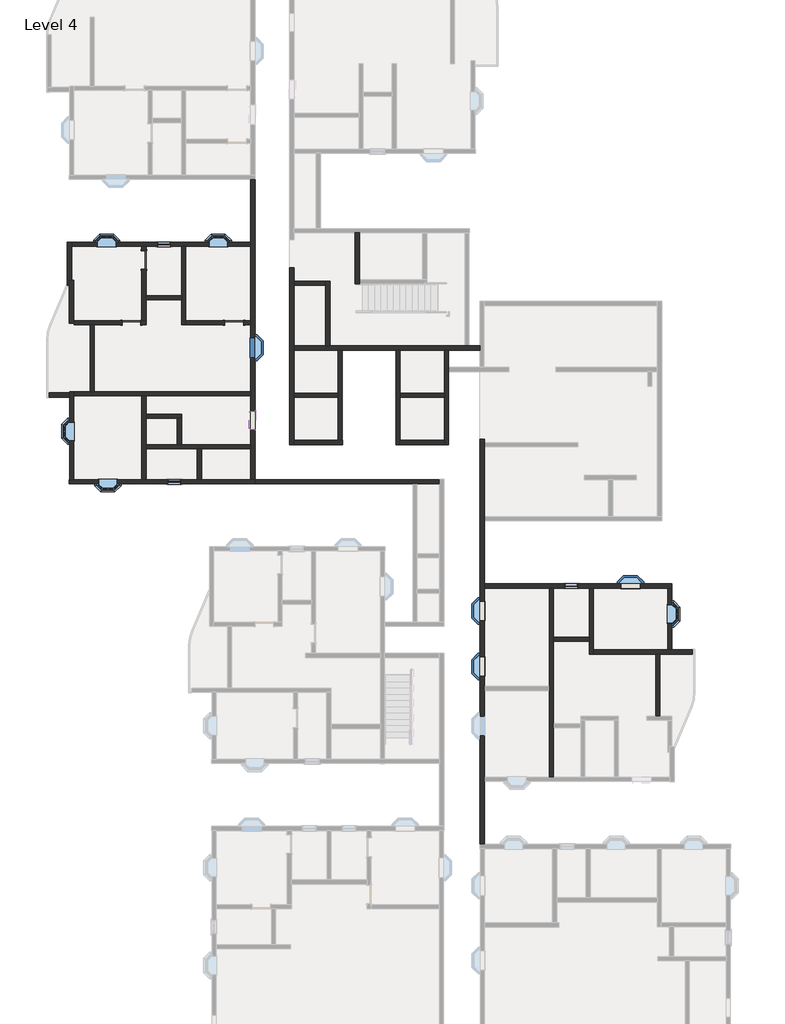
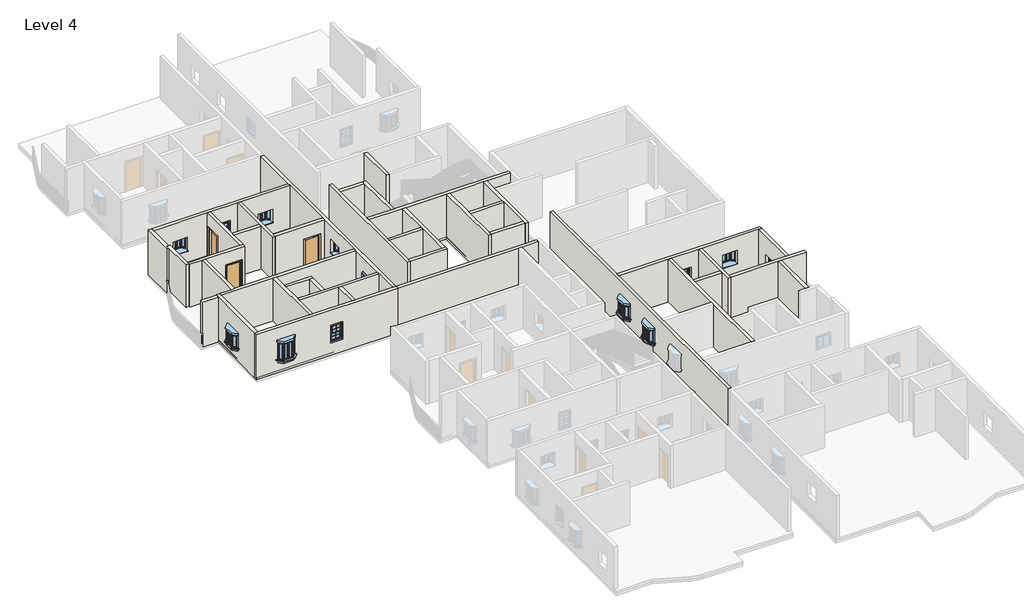
# One storey, part 3 of 14: 40 walls, 13 windows, 3 doors.
# Revit data of these elements (continued)
# Element 26 (IfcWall, "9\"")
#   Top Offset = 0' - 0"
#   Base Offset = 0' - 0"
#   wall height = 10' - 0"
#   Phase Created = New Construction
#   Base Constraint = Level 4
#   Top Constraint = Level 5
#   Materials on its faces: "Earth", "Default Wall"
# Element 27 (IfcWall, "9\"")
#   Top Offset = 0' - 0"
#   Base Offset = 0' - 0"
#   wall height = 10' - 0"
#   Phase Created = New Construction
#   Base Constraint = Level 4
#   Top Constraint = Level 5
#   Materials on its faces: "Default Wall", "Default Mass Interior Wall"
# Element 28 (IfcWall, "9\"")
#   Top Offset = 0' - 0"
#   Base Offset = 0' - 0"
#   wall height = 10' - 0"
#   Phase Created = New Construction
#   Base Constraint = Level 4
#   Top Constraint = Level 5
#   Materials on its faces: "Default Wall"
# Element 29 (IfcWall, "9\"")
#   Top Offset = 0' - 0"
#   Base Offset = 0' - 0"
#   wall height = 10' - 0"
#   Phase Created = New Construction
#   Base Constraint = Level 4
#   Top Constraint = Level 5
#   Materials on its faces: "Default Wall", "Default Mass Interior Wall", "Earth"
# Elements 30, 33, 34, 35, 36, 37, 38, 39, 40, 41 (IfcWall, "9\" w")
#   Top Offset = 0' - 0"
#   Base Offset = 0' - 0"
#   wall height = 10' - 0"
#   Phase Created = New Construction
#   Base Constraint = Level 4
#   Top Constraint = Level 5
#   Materials on its faces: "Default Wall"
# Element 31 (IfcWall, "9\" w")
#   Top Offset = 0' - 0"
#   Base Offset = 0' - 0"
#   wall height = 10' - 0"
#   Phase Created = New Construction
#   Base Constraint = Level 4
#   Top Constraint = Level 5
#   Materials on its faces: "Default Wall", "Earth"
# Element 32 (IfcWall, "9\" w")
#   Top Offset = 0' - 0"
#   Base Offset = 0' - 0"
#   wall height = 10' - 0"
#   Phase Created = New Construction
#   Base Constraint = Level 4
#   Top Constraint = Level 5
#   Materials on its faces: "Default Wall", "Brick, Soldier Course"
# Element 42 (IfcWall, "9\" w")
#   Top Offset = 0' - 0"
#   Base Offset = 0' - 0"
#   wall height = 10' - 0"
#   Phase Created = New Construction
#   Base Constraint = Level 4
#   Top Constraint = Level 5
#   Materials on its faces: "Default Wall", "Wood - Stained"
# Element 43 (IfcWall, "9\" w")
#   Top Offset = 0' - 0"
#   Base Offset = 0' - 0"
#   wall height = 10' - 0"
#   Phase Created = New Construction
#   Base Constraint = Level 4
#   Top Constraint = Level 5
#   Materials on its faces: "Default Wall", "Acoustic Ceiling Tile 24 x 24"
# Element 44 (IfcWindow, "910x1210mm")
#   Mark = "305"
#   Phase Created = New Construction
#   Materials on its faces: "Window Frame", "Glass"
# Element 45 (IfcWindow, "910x910mm")
#   Mark = "199"
#   Phase Created = New Construction
#   Materials on its faces: "Window Frame", "Glass"
# Element 46 (IfcWindow, "910x910mm")
#   Mark = "200"
#   Phase Created = New Construction
#   Materials on its faces: "Window Frame", "Glass"
# Element 47 (IfcWindow, "910x910mm")
#   Mark = "172"
#   Phase Created = New Construction
#   Materials on its faces: "Window Frame", "Glass"
# Element 48 (IfcWindow, "910x910mm")
#   Mark = "173"
#   Phase Created = New Construction
#   Materials on its faces: "Window Frame", "Glass"
# Element 49 (IfcWindow, "910x910mm")
#   Mark = "174"
#   Phase Created = New Construction
#   Materials on its faces: "Window Frame", "Glass"
# Element 50 (IfcWindow, "910x910mm")
#   Mark = "175"
#   Phase Created = New Construction
#   Materials on its faces: "Window Frame", "Glass"
# Element 51 (IfcWindow, "910x910mm")
#   Mark = "197"
#   Phase Created = New Construction
#   Materials on its faces: "Window Frame", "Glass"
# Element 52 (IfcWindow, "910x910mm")
#   Mark = "198"
#   Phase Created = New Construction
#   Materials on its faces: "Window Frame", "Glass"
# Element 53 (IfcWindow, "Window-Double-Hung : 26\" x 42\"")
#   Mark = "221"
#   Window Inset = 0' - 0"
#   Interior Wall Closure = 0' - 1 1/2"
#   Frame Extension = 0' - 1 1/4"
#   Exterior Wall Closure = 0' - 0 1/2"
#   Interior Trim Visibility = yes
#   Indicator Visibility = yes
#   Exterior Trim Visibility = yes
#   Phase Created = New Construction
#   Materials on its faces: "Wood - Stained", "Glass", "Clad - White"
# Element 54 (IfcWindow, "Window-Double-Hung : 26\" x 42\"")
#   Mark = "210"
#   Window Inset = 0' - 0"
#   Interior Wall Closure = 0' - 1 1/2"
#   Frame Extension = 0' - 1 1/4"
#   Exterior Wall Closure = 0' - 0 1/2"
#   Interior Trim Visibility = yes
#   Indicator Visibility = yes
#   Exterior Trim Visibility = yes
#   Phase Created = New Construction
#   Materials on its faces: "Wood - Stained", "Glass", "Clad - White"
# Element 55 (IfcWindow, "Window-Double-Hung : 26\" x 42\"")
#   Mark = "211"
#   Window Inset = 0' - 0"
#   Interior Wall Closure = 0' - 1 1/2"
#   Frame Extension = 0' - 1 1/4"
#   Exterior Wall Closure = 0' - 0 1/2"
#   Interior Trim Visibility = yes
#   Indicator Visibility = yes
#   Exterior Trim Visibility = yes
#   Phase Created = New Construction
#   Materials on its faces: "Wood - Stained", "Glass", "Clad - White"
# Element 56 (IfcWindow, "Windows_Sgl_w-Glazing_Bars : 910x910mm")
#   Mark = "206"
#   Phase Created = New Construction
#   Materials on its faces: "Window Frame", "Glass"
# Materials
#   "Door - Panel": class "Wood", colour RGB 210 159 95, transparency 0, Cost = 0
#   "Door - Frame": colour RGB 118 70 51, transparency 0, Cost = 0
#   "Window Frame": colour RGB 249 249 249, transparency 0
#   "Glass": class "Glass", colour RGB 0 128 192, transparency 0.75, Description = "Soda Lime Glass", Cost = 0
#   "Wood - Stained": class "Wood", colour RGB 224 178 126, transparency 0, Cost = 0
#   "Clad - White": class "Wood", colour RGB 242 242 238, transparency 0, Cost = 0
#   "Default Wall": colour RGB 128 128 128, transparency 0, Cost = 0
#   "Cherry": class "Wood", colour RGB 226 177 128, transparency 0, Description = "Prunus Serotina", Cost = 0
#   "Parking Stripe": class "Paint", colour RGB 250 250 91, transparency 0, Cost = 0
#   "Earth": class "Generic", colour RGB 97 75 62, transparency 0, Description = "Soil", Cost = 0
#   "Default Mass Interior Wall": class "Generic", colour RGB 195 229 126, transparency 0, Cost = 0
#   "Brick, Soldier Course": class "Masonry", colour RGB 170 98 104, transparency 0, Description = "Common brick soldier coursed", Cost = 0
#   "Acoustic Ceiling Tile 24 x 24": class "Generic", colour RGB 232 232 232, transparency 0, Description = "Acoustic Ceiling Tile 24 x 24", Cost = 0
